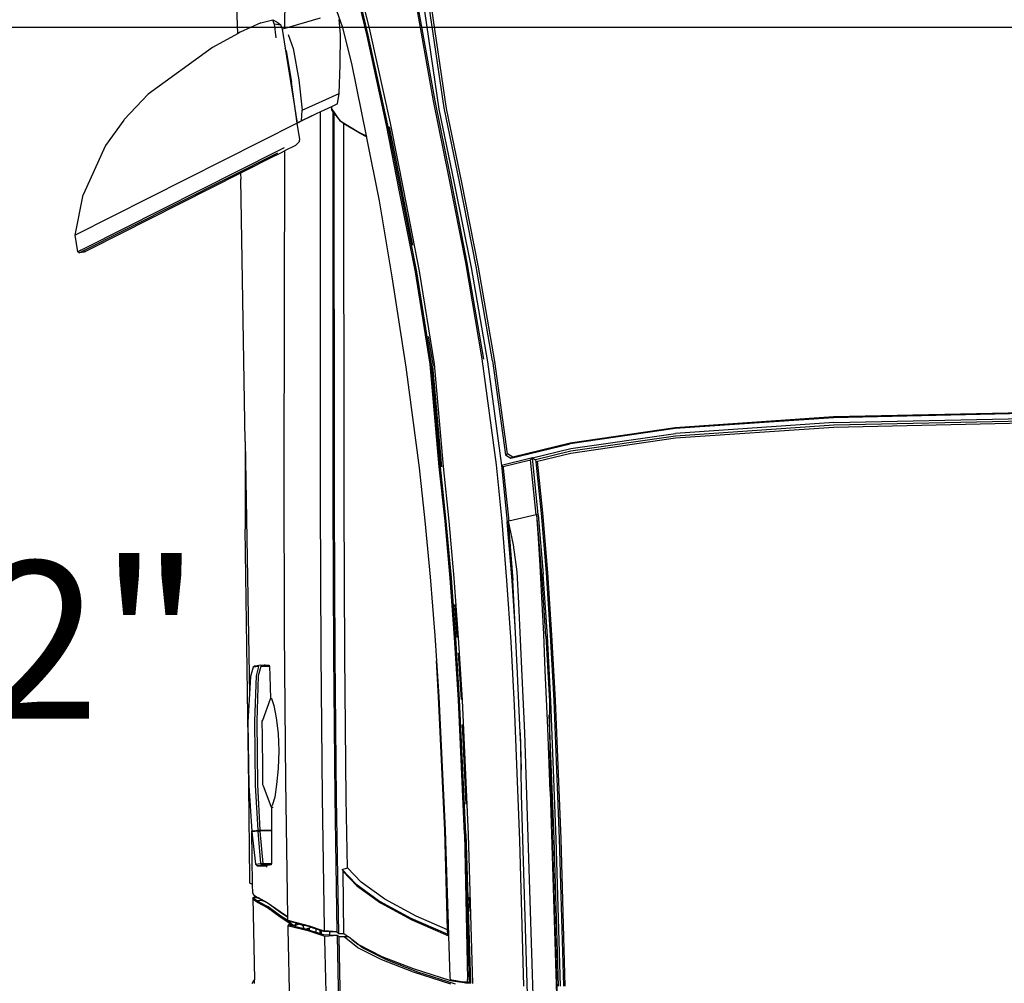
# Model space of a CAD drawing. Units: inches. Extents: x 1319 to 2030, y 219 to 1069.
# Tile 10 of 28: x 1417 to 1461, y 430 to 473. Entities that reach past the tile are written whole.
import ezdxf

# ---------------------------------------------------------------- set-up
doc = ezdxf.new("R2010")
doc.units = ezdxf.units.IN
doc.header["$MEASUREMENT"] = 0
doc.layers.get('0').update_dxf_attribs({"color": 12})
doc.layers.add('A-ANNO-DIMS', color=2, linetype='Continuous', lineweight=18)
doc.layers.add('C-PRKG-VEHC', color=8, linetype='Continuous', lineweight=13)
doc.layers.add('Edges', color=250, linetype='Continuous')
doc.styles.get("Standard").update_dxf_attribs({"font": 'arial.ttf'})
doc.dimstyles.get("Standard").update_dxf_attribs({"dimtxt": 7, "dimasz": 0.18, "dimexe": 0.18, "dimexo": 0.0625, "dimgap": 0.09, "dimtad": 0, "dimtih": 1, "dimtoh": 1, "dimzin": 0, "dimdsep": 46, "dimlunit": 3, "dimtxsty": 'Standard', "dimcen": 0.09, "dimadec": 0, "dimazin": 0, "dimtfac": 1, "dimtofl": 0, "dimtmove": 0, "dimatfit": 3, "dimfxl": 1, "dimtolj": 1, "dimtzin": 0, "dimarcsym": 0})

# ---------------------------------------------------------------- blocks, each defined once
blk = doc.blocks.new('Nissan Qashqai pl')
at = {"layer": 'Edges'}
for p, q in [((9.2195, 11.9221), (9.2241, 11.7066)), ((9.2203, 11.9221), (9.2249, 11.7065)), ((9.2305, 11.7067), (9.2259, 11.9221)), ((9.2289, 11.9221), (9.2335, 11.7067)), ((9.2355, 11.7068), (9.2308, 11.9221)), ((9.2241, 11.7066), (9.2362, 11.5274)), ((9.2249, 11.7065), (9.2371, 11.5273)), ((9.2305, 11.7067), (9.2426, 11.5277)), ((9.2335, 11.7067), (9.2457, 11.5277)), ((9.2476, 11.5278), (9.2355, 11.7068)), ((9.2362, 11.5274), (9.2535, 11.4087)), ((9.2371, 11.5273), (9.2543, 11.4085)), ((9.2598, 11.4093), (9.2426, 11.5277)), ((9.2457, 11.5277), (9.2629, 11.4092)), ((9.2649, 11.4094), (9.2476, 11.5278)), ((9.2535, 11.4087), (9.2694, 11.3436)), ((9.2707, 11.3414), (9.2543, 11.4085)), ((9.2704, 11.3659), (9.2598, 11.4093)), ((9.2629, 11.4092), (9.2726, 11.3695)), ((9.2741, 11.3716), (9.2649, 11.4094)), ((9.701, 11.3983), (9.5443, 11.3919)), ((9.5446, 11.39), (9.7011, 11.3963)), ((9.7014, 11.3929), (9.5454, 11.3866)), ((9.6472, 11.3861), (9.9278, 11.3949)), ((9.6714, 11.3874), (9.8565, 11.3931)), ((9.8673, 11.4031), (9.701, 11.3983)), ((9.7011, 11.3963), (9.8673, 11.4012)), ((9.8673, 11.3977), (9.7014, 11.3929)), ((9.8673, 11.3954), (9.7014, 11.3906)), ((9.8565, 11.3931), (9.9794, 11.3967)), ((9.4, 11.3832), (9.3326, 11.3776)), ((9.333, 11.3757), (9.4004, 11.3813)), ((9.4706, 11.388), (9.4, 11.3832)), ((9.4004, 11.3813), (9.4709, 11.3861)), ((9.472, 11.3812), (9.4017, 11.3765)), ((9.472, 11.3828), (9.4018, 11.378)), ((9.5443, 11.3919), (9.4706, 11.388)), ((9.4709, 11.3861), (9.5446, 11.39)), ((9.5454, 11.3866), (9.472, 11.3828)), ((9.472, 11.3812), (9.5454, 11.3851)), ((9.5755, 11.3834), (9.5105, 11.3805)), ((9.5454, 11.3851), (9.5695, 11.3853)), ((9.5454, 11.3848), (9.5454, 11.3851)), ((9.5695, 11.3853), (9.5609, 11.3849)), ((9.7014, 11.3906), (9.5695, 11.3853)), ((9.5695, 11.3853), (9.5786, 11.3853)), ((9.6472, 11.3861), (9.5755, 11.3834)), ((9.5786, 11.3853), (9.6206, 11.3861)), ((9.6206, 11.3861), (9.6714, 11.3874)), ((9.3346, 11.3724), (9.2704, 11.3659)), ((9.3346, 11.37), (9.2724, 11.3637)), ((9.3326, 11.3776), (9.2741, 11.3716)), ((9.2746, 11.3697), (9.333, 11.3757)), ((9.4017, 11.3765), (9.3344, 11.3708)), ((9.3611, 11.3727), (9.3344, 11.3708)), ((9.3344, 11.3708), (9.3346, 11.37)), ((9.3346, 11.3724), (9.4018, 11.378)), ((9.3346, 11.37), (9.3418, 11.3391)), ((9.3918, 11.3747), (9.3611, 11.3727)), ((9.4276, 11.3767), (9.3918, 11.3747)), ((9.4694, 11.3788), (9.4276, 11.3767)), ((9.5105, 11.3805), (9.4694, 11.3788)), ((9.2704, 11.3659), (9.2726, 11.3695)), ((9.2704, 11.3659), (9.2724, 11.3637)), ((9.2704, 11.3659), (9.2789, 11.331)), ((9.2799, 11.3328), (9.2724, 11.3637)), ((9.2726, 11.3695), (9.2746, 11.3697)), ((9.5812, 11.3568), (9.6514, 11.3592)), ((9.9583, 11.363), (9.651, 11.3536)), ((9.6514, 11.3592), (9.9312, 11.3681)), ((9.3687, 11.3441), (9.3992, 11.3482)), ((9.3992, 11.3482), (9.4347, 11.3502)), ((9.4347, 11.3502), (9.4761, 11.3522)), ((9.514, 11.3492), (9.4605, 11.3465)), ((9.4761, 11.3522), (9.5168, 11.3539)), ((9.5811, 11.3522), (9.514, 11.3492)), ((9.5168, 11.3539), (9.5812, 11.3568)), ((9.7029, 11.3516), (9.5503, 11.3455)), ((9.5811, 11.3522), (9.6231, 11.3531)), ((9.594, 11.3527), (9.5811, 11.3522)), ((9.6231, 11.3531), (9.594, 11.3527)), ((9.651, 11.3536), (9.6231, 11.3531)), ((9.8673, 11.3563), (9.7029, 11.3516)), ((9.2656, 11.3376), (9.1612, 11.3233)), ((9.2694, 11.3436), (9.2656, 11.3376)), ((9.2669, 11.3354), (9.2656, 11.3376)), ((9.2669, 11.3354), (9.2707, 11.3414)), ((9.2694, 11.3436), (9.2707, 11.3414)), ((9.2789, 11.331), (9.3427, 11.3375)), ((9.2819, 11.333), (9.3418, 11.3391)), ((9.3418, 11.3391), (9.342, 11.3383)), ((9.342, 11.3383), (9.3687, 11.3441)), ((9.342, 11.3383), (9.4087, 11.3438)), ((9.4088, 11.3371), (9.3422, 11.3316)), ((9.4093, 11.3431), (9.3427, 11.3375)), ((9.4605, 11.3465), (9.4087, 11.3438)), ((9.4782, 11.3418), (9.4088, 11.3371)), ((9.4605, 11.3465), (9.4093, 11.3431)), ((9.5503, 11.3455), (9.4782, 11.3418)), ((9.1605, 11.3208), (9.2669, 11.3354)), ((9.1617, 11.315), (9.2789, 11.331)), ((9.3422, 11.3316), (9.2783, 11.3251)), ((9.2789, 11.331), (9.2799, 11.3327)), ((9.2799, 11.3328), (9.2819, 11.333)), ((9.2799, 11.3327), (9.2799, 11.3328)), ((9.2799, 11.3327), (9.2811, 11.3325)), ((9.1605, 11.3208), (9.0538, 11.3023)), ((9.1612, 11.3233), (9.0546, 11.3048)), ((9.0552, 11.2965), (9.1617, 11.315)), ((9.2783, 11.3251), (9.1584, 11.3091)), ((9.0546, 11.3048), (8.9591, 11.2859)), ((9.1584, 11.3091), (9.0495, 11.2906)), ((9.0497, 11.2918), (9.1586, 11.3104)), ((9.0538, 11.3023), (8.9583, 11.2833)), ((8.9598, 11.2775), (9.0552, 11.2965)), ((9.5443, 11.2863), (9.696, 11.2932)), ((9.6953, 11.2892), (9.863, 11.2944)), ((9.6953, 11.2892), (9.8598, 11.2925)), ((9.6954, 11.2907), (9.8641, 11.2959)), ((9.696, 11.2932), (9.8644, 11.2982)), ((9.7669, 11.2945), (9.7832, 11.2951)), ((9.8629, 11.2925), (9.8598, 11.2925)), ((9.8627, 11.2909), (9.8629, 11.2925)), ((9.8629, 11.2925), (9.863, 11.2944)), ((9.8641, 11.2959), (9.863, 11.2944)), ((9.8637, 11.291), (9.8638, 11.2934)), ((9.8638, 11.2934), (9.8641, 11.2959)), ((8.9583, 11.2833), (8.8745, 11.266)), ((8.9591, 11.2859), (8.8754, 11.2687)), ((9.0495, 11.2906), (8.9521, 11.2715)), ((8.9522, 11.2728), (9.0497, 11.2918)), ((9.4064, 11.277), (9.4739, 11.282)), ((9.5437, 11.2822), (9.4735, 11.2779)), ((9.5438, 11.2836), (9.4736, 11.2793)), ((9.4739, 11.282), (9.5443, 11.2863)), ((9.491, 11.2819), (9.5434, 11.2852)), ((9.6953, 11.2892), (9.5437, 11.2822)), ((9.6954, 11.2907), (9.5438, 11.2836)), ((9.5717, 11.2865), (9.6618, 11.2907)), ((9.8605, 11.2746), (9.8626, 11.2878)), ((9.8615, 11.2754), (9.8635, 11.2886)), ((9.8626, 11.2878), (9.8627, 11.2909)), ((9.8627, 11.2909), (9.8637, 11.291)), ((9.8635, 11.2886), (9.8637, 11.291)), ((9.8637, 11.291), (9.8643, 11.291)), ((8.8666, 11.2554), (8.9522, 11.2728)), ((8.9521, 11.2715), (8.8666, 11.2541)), ((8.8761, 11.2602), (8.9598, 11.2775)), ((9.2801, 11.2648), (9.3418, 11.2713)), ((9.3418, 11.2713), (9.4064, 11.277)), ((9.4062, 11.2729), (9.3418, 11.2671)), ((9.4063, 11.2743), (9.3419, 11.2685)), ((9.4735, 11.2779), (9.4062, 11.2729)), ((9.4736, 11.2793), (9.4063, 11.2743)), ((9.4727, 11.2808), (9.4362, 11.278)), ((9.4727, 11.2808), (9.4732, 11.2808)), ((9.8039, 11.27), (9.6912, 11.2667)), ((9.6913, 11.2674), (9.8099, 11.2711)), ((9.8039, 11.27), (9.7884, 11.2343)), ((9.7905, 11.2283), (9.8087, 11.2702)), ((9.7925, 11.2294), (9.8107, 11.2711)), ((9.8087, 11.2702), (9.8039, 11.27)), ((9.8099, 11.2711), (9.8087, 11.2702)), ((9.8099, 11.2711), (9.8107, 11.2711)), ((9.8107, 11.2711), (9.8573, 11.2726)), ((9.8475, 11.2312), (9.8611, 11.2734)), ((9.8652, 11.2788), (9.8516, 11.2363)), ((9.8652, 11.2738), (9.8516, 11.2313)), ((9.8573, 11.2726), (9.8603, 11.2727)), ((9.8603, 11.2727), (9.8605, 11.2746)), ((9.8611, 11.2734), (9.8603, 11.2727)), ((9.8612, 11.2735), (9.8611, 11.2734)), ((9.8612, 11.2735), (9.8615, 11.2754)), ((8.8745, 11.266), (8.7481, 11.2473)), ((8.8754, 11.2687), (8.7491, 11.2501)), ((8.7496, 11.2416), (8.8761, 11.2602)), ((9.1639, 11.2546), (9.2801, 11.2648)), ((9.2803, 11.2606), (9.1644, 11.2503)), ((9.2804, 11.262), (9.1645, 11.2518)), ((9.2804, 11.2635), (9.1668, 11.2533)), ((9.3418, 11.2671), (9.2803, 11.2606)), ((9.3419, 11.2685), (9.2804, 11.262)), ((9.4997, 11.2573), (9.5403, 11.26)), ((9.5404, 11.2598), (9.4997, 11.2573)), ((9.5403, 11.26), (9.6913, 11.2674)), ((9.6912, 11.2667), (9.5404, 11.2598)), ((8.7287, 11.2307), (8.8666, 11.2554)), ((8.8666, 11.2541), (8.7292, 11.2295)), ((9.0591, 11.2377), (9.1639, 11.2546)), ((9.1644, 11.2503), (9.06, 11.2335)), ((9.1645, 11.2518), (9.0601, 11.235)), ((9.133, 11.2481), (9.1647, 11.2532)), ((9.1647, 11.2532), (9.1668, 11.2533)), ((9.3416, 11.2442), (9.4048, 11.2501)), ((9.4048, 11.2501), (9.471, 11.2554)), ((9.471, 11.2554), (9.4997, 11.2573)), ((8.9679, 11.2201), (9.0591, 11.2377)), ((9.1676, 11.2229), (9.2814, 11.2377)), ((9.2814, 11.2377), (9.3416, 11.2442)), ((9.0601, 11.235), (8.8941, 11.2023)), ((9.06, 11.2335), (8.9696, 11.2157)), ((8.9708, 11.2185), (9.03, 11.2304)), ((9.7884, 11.2343), (9.7692, 11.1989)), ((9.7713, 11.1929), (9.7905, 11.2283)), ((9.7733, 11.194), (9.7925, 11.2294)), ((9.8338, 11.1956), (9.8475, 11.2312)), ((9.8516, 11.2363), (9.8378, 11.2007)), ((9.8516, 11.2313), (9.8378, 11.1957)), ((8.8918, 11.205), (8.9679, 11.2201)), ((8.9696, 11.2157), (8.8942, 11.2009)), ((8.9318, 11.211), (8.9704, 11.2185)), ((8.9704, 11.2185), (8.9708, 11.2185)), ((9.0656, 11.207), (9.1676, 11.2229)), ((8.7881, 11.1821), (8.8918, 11.205)), ((8.8961, 11.204), (8.9318, 11.211)), ((8.9797, 11.1924), (9.0656, 11.207)), ((8.8941, 11.2023), (8.7925, 11.1802)), ((8.8942, 11.2009), (8.7931, 11.1789)), ((8.9087, 11.1783), (8.9797, 11.1924)), ((9.7692, 11.1989), (9.7499, 11.1721)), ((9.7519, 11.1661), (9.7713, 11.1929)), ((9.754, 11.1672), (9.7733, 11.194)), ((9.8201, 11.1685), (9.8338, 11.1956)), ((9.8378, 11.2007), (9.8241, 11.1736)), ((9.8378, 11.1957), (9.8241, 11.1686)), ((8.7575, 11.1744), (8.7881, 11.1821)), ((8.7931, 11.1789), (8.7574, 11.1704)), ((8.7925, 11.1802), (8.7591, 11.1723)), ((8.8245, 11.1613), (8.9063, 11.1779)), ((8.8893, 11.1486), (8.9021, 11.1697)), ((8.9041, 11.1717), (8.8927, 11.1528)), ((8.9021, 11.1697), (8.9063, 11.1779)), ((8.9075, 11.1781), (8.9041, 11.1717)), ((8.9063, 11.1779), (8.9075, 11.1781)), ((8.9075, 11.1781), (8.9087, 11.1783)), ((9.7499, 11.1721), (9.7337, 11.1566)), ((9.8241, 11.1736), (9.8147, 11.1616)), ((8.7828, 11.1508), (8.8245, 11.1613)), ((9.7357, 11.1507), (9.7519, 11.1661)), ((9.7378, 11.1517), (9.754, 11.1672)), ((9.8241, 11.1686), (9.8119, 11.1529)), ((9.8147, 11.1616), (9.8119, 11.1579)), ((9.8147, 11.1616), (9.8201, 11.1685)), ((9.8147, 11.1616), (9.8147, 11.1616)), ((8.7524, 11.1401), (8.7828, 11.1508)), ((8.7916, 11.1488), (8.7748, 11.1475)), ((8.8259, 11.1483), (8.7916, 11.1488)), ((8.8585, 11.1473), (8.8259, 11.1483)), ((8.87, 11.1455), (8.8585, 11.1473)), ((8.8771, 11.1054), (8.8585, 11.1473)), ((8.8893, 11.1486), (8.8751, 11.1387)), ((8.881, 11.1418), (8.8893, 11.1486)), ((8.8913, 11.1506), (8.8893, 11.1486)), ((8.8927, 11.1528), (8.8913, 11.1506)), ((9.3225, 11.1531), (8.8927, 11.1528)), ((9.4936, 11.1538), (9.3225, 11.1531)), ((9.6552, 11.1554), (9.4936, 11.1538)), ((9.7337, 11.1566), (9.6552, 11.1554)), ((9.7357, 11.1507), (9.7337, 11.1566)), ((9.7357, 11.1507), (9.7378, 11.1517)), ((9.8078, 11.1528), (9.7378, 11.1517)), ((9.8078, 11.1528), (9.8119, 11.1579)), ((9.8078, 11.1471), (9.8078, 11.1528)), ((9.8101, 11.1449), (9.9411, 11.1475)), ((9.8119, 11.1579), (9.8119, 11.1529)), ((9.8119, 11.1529), (9.8119, 11.1472)), ((9.9393, 11.1497), (9.8119, 11.1472)), ((8.87, 11.1455), (8.8734, 11.1385)), ((8.8734, 11.1385), (8.8793, 11.1261)), ((8.8734, 11.1385), (8.8768, 11.1385)), ((8.8751, 11.1387), (8.8768, 11.1385)), ((8.8768, 11.1385), (8.879, 11.1402)), ((8.879, 11.1402), (8.881, 11.1418)), ((8.879, 11.1402), (9.3198, 11.1403)), ((9.3225, 11.1421), (8.881, 11.1418)), ((9.3198, 11.1403), (9.4922, 11.1409)), ((9.4936, 11.1428), (9.3225, 11.1421)), ((9.4922, 11.1409), (9.654, 11.1423)), ((9.6552, 11.1445), (9.4936, 11.1428)), ((9.654, 11.1423), (9.8061, 11.1447)), ((9.8078, 11.1471), (9.6552, 11.1445)), ((9.8061, 11.1447), (9.8051, 11.1309)), ((9.8055, 11.1298), (9.8058, 11.1369)), ((9.8058, 11.1369), (9.8061, 11.1447)), ((9.8098, 11.1369), (9.8058, 11.1369)), ((9.8061, 11.1447), (9.8078, 11.1471)), ((9.8098, 11.1369), (9.8096, 11.13)), ((9.8101, 11.1449), (9.8098, 11.1369)), ((9.8119, 11.1472), (9.8101, 11.1449)), ((9.8101, 11.1449), (9.8112, 11.1311)), ((8.7733, 11.126), (8.7849, 11.0859)), ((9.3194, 11.1262), (8.8793, 11.1261)), ((8.8793, 11.1261), (8.8815, 11.1214)), ((9.4919, 11.1269), (9.3194, 11.1262)), ((9.6538, 11.1284), (9.4919, 11.1269)), ((9.802, 11.1309), (9.6538, 11.1284)), ((9.7992, 11.1133), (9.8044, 11.129)), ((9.8051, 11.1309), (9.802, 11.1309)), ((9.8026, 11.1212), (9.8041, 11.1256)), ((9.8041, 11.1256), (9.8045, 11.1268)), ((9.8041, 11.1256), (9.8081, 11.1256)), ((9.8044, 11.129), (9.8051, 11.1309)), ((9.8045, 11.1268), (9.8046, 11.1271)), ((9.8045, 11.1268), (9.8085, 11.1268)), ((9.8046, 11.1271), (9.8055, 11.1298)), ((9.8086, 11.1271), (9.8046, 11.1271)), ((9.8106, 11.1292), (9.8054, 11.1135)), ((9.8081, 11.1256), (9.8067, 11.1213)), ((9.8085, 11.1268), (9.8081, 11.1256)), ((9.8086, 11.1271), (9.8085, 11.1268)), ((9.8096, 11.13), (9.8086, 11.1271)), ((9.8112, 11.1311), (9.8106, 11.1292)), ((9.8143, 11.1312), (9.8112, 11.1311)), ((9.9414, 11.1341), (9.8143, 11.1312)), ((8.8815, 11.1214), (8.892, 11.0998)), ((8.8815, 11.1214), (8.8895, 11.1048)), ((9.7987, 11.108), (9.8002, 11.1141)), ((9.8002, 11.1141), (9.8008, 11.1157)), ((9.8008, 11.1157), (9.8014, 11.1176)), ((9.8014, 11.1139), (9.8008, 11.1157)), ((9.803, 11.1212), (9.8014, 11.1176)), ((9.8014, 11.1176), (9.8026, 11.1212)), ((9.8043, 11.1139), (9.8014, 11.1139)), ((9.8031, 11.1093), (9.8014, 11.1139)), ((9.803, 11.1212), (9.8026, 11.1212)), ((9.8067, 11.1213), (9.803, 11.1212)), ((9.8043, 11.1139), (9.8031, 11.1093)), ((9.8044, 11.1142), (9.8043, 11.1139)), ((9.8067, 11.1213), (9.8044, 11.1142)), ((8.8429, 11.1016), (8.8771, 11.1054)), ((8.8895, 11.1048), (8.8771, 11.1054)), ((8.8908, 11.1021), (8.8895, 11.1048)), ((8.8906, 11.1024), (8.8895, 11.1048)), ((8.9106, 11.1029), (8.892, 11.0998)), ((8.9131, 11.102), (8.9106, 11.1029)), ((9.7937, 11.0918), (9.7992, 11.1133)), ((9.7973, 11.1023), (9.7977, 11.1042)), ((9.7977, 11.1033), (9.7973, 11.1023)), ((9.7987, 11.1053), (9.7977, 11.1033)), ((9.7977, 11.1042), (9.7978, 11.1044)), ((9.7977, 11.1042), (9.7977, 11.1033)), ((9.7978, 11.1044), (9.7987, 11.108)), ((9.7987, 11.1053), (9.7978, 11.1044)), ((9.7992, 11.1065), (9.7987, 11.108)), ((9.7992, 11.1065), (9.7987, 11.1053)), ((9.8027, 11.1078), (9.7992, 11.1065)), ((9.8054, 11.1135), (9.7999, 11.0919)), ((9.8027, 11.1078), (9.8003, 11.0983)), ((9.8031, 11.1093), (9.8027, 11.1078)), ((8.7917, 11.0895), (8.8075, 11.0955)), ((8.807, 11.0862), (8.8918, 11.0997)), ((8.8075, 11.0955), (8.8429, 11.1016)), ((8.8102, 11.0874), (8.8455, 11.0936)), ((8.8918, 11.0997), (8.8455, 11.0936)), ((8.8906, 11.1024), (8.8911, 11.1013)), ((8.892, 11.0998), (8.8908, 11.1021)), ((8.8911, 11.1013), (8.8919, 11.0997)), ((8.8911, 11.1013), (8.8919, 11.0998)), ((8.8919, 11.0997), (8.8911, 11.1013)), ((8.8919, 11.0997), (8.8918, 11.0997)), ((8.8918, 11.0997), (9.0186, 10.8486)), ((8.892, 11.0998), (8.8919, 11.0998)), ((8.8919, 11.0998), (8.8919, 11.0997)), ((8.8919, 11.0997), (8.8919, 11.0997)), ((8.892, 11.0998), (8.892, 11.0998)), ((8.9171, 11.0978), (8.9131, 11.102)), ((8.9171, 11.0978), (8.917, 11.0974)), ((8.9171, 11.0978), (8.9233, 11.0855)), ((9.7965, 11.0915), (9.7894, 11.0806)), ((9.7934, 11.0906), (9.7937, 11.0918)), ((9.7964, 11.0988), (9.7943, 11.0907)), ((9.7955, 11.0925), (9.7943, 11.0907)), ((9.7963, 11.0918), (9.7955, 11.0925)), ((9.7992, 11.0966), (9.7963, 11.0918)), ((9.7963, 11.0918), (9.7963, 11.0918)), ((9.7964, 11.0917), (9.7963, 11.0918)), ((9.7964, 11.0988), (9.7973, 11.1023)), ((9.7964, 11.0988), (9.7992, 11.0966)), ((9.7964, 11.0917), (9.7996, 11.0966)), ((9.7964, 11.0917), (9.7964, 11.0917)), ((9.7967, 11.0915), (9.7964, 11.0917)), ((9.7965, 11.0915), (9.7967, 11.0915)), ((9.7983, 11.0901), (9.7965, 11.0915)), ((9.7967, 11.0915), (9.7986, 11.0916)), ((9.7977, 11.0907), (9.7967, 11.0915)), ((9.7973, 11.1023), (9.7977, 11.1011)), ((9.7977, 11.1011), (9.7977, 11.0998)), ((9.7977, 11.1011), (9.7985, 11.099)), ((9.7977, 11.0998), (9.7985, 11.099)), ((9.7986, 11.0916), (9.7982, 11.0902)), ((9.7985, 11.099), (9.7989, 11.098)), ((9.7988, 11.0925), (9.7986, 11.0916)), ((9.7998, 11.0964), (9.7988, 11.0925)), ((9.7989, 11.098), (9.7998, 11.0976)), ((9.7998, 11.0976), (9.7992, 11.0966)), ((9.7999, 11.0919), (9.7993, 11.0891)), ((9.8002, 11.098), (9.7996, 11.0966)), ((9.8001, 11.0974), (9.7996, 11.0966)), ((9.7996, 11.0966), (9.7998, 11.0964)), ((9.8003, 11.0983), (9.7998, 11.0976)), ((9.8001, 11.0974), (9.7998, 11.0964)), ((9.8002, 11.098), (9.8001, 11.0974)), ((9.8003, 11.0983), (9.8002, 11.098)), ((9.8024, 11.0892), (9.9426, 11.0923)), ((8.7849, 11.0859), (8.7205, 11.0863)), ((8.7779, 11.0773), (8.7807, 11.0812)), ((8.7798, 11.0739), (8.7807, 11.0812)), ((8.7849, 11.0827), (8.7807, 11.0812)), ((8.7849, 11.0859), (8.7856, 11.0834)), ((8.7849, 11.0827), (8.7858, 11.0828)), ((8.7858, 11.0828), (8.7856, 11.0834)), ((8.7858, 11.0828), (8.807, 11.0862)), ((8.8102, 11.0874), (8.807, 11.0862)), ((8.9232, 11.0779), (8.9194, 11.0854)), ((8.9233, 11.0855), (9.2886, 11.0848)), ((8.925, 11.0821), (8.9233, 11.0855)), ((8.928, 11.0762), (8.925, 11.0821)), ((9.2886, 11.0848), (9.4673, 11.0852)), ((9.4673, 11.0852), (9.6358, 11.0866)), ((9.6358, 11.0866), (9.7887, 11.0889)), ((9.7728, 11.066), (9.7832, 11.0805)), ((9.7738, 11.067), (9.7842, 11.0814)), ((9.7883, 11.0815), (9.7778, 11.0671)), ((9.7894, 11.0806), (9.7788, 11.0661)), ((9.7832, 11.0805), (9.7887, 11.0889)), ((9.7842, 11.0814), (9.7891, 11.0889)), ((9.7933, 11.0892), (9.7883, 11.0815)), ((9.7887, 11.0889), (9.7891, 11.0889)), ((9.7891, 11.0889), (9.79, 11.0889)), ((9.79, 11.0889), (9.7931, 11.089)), ((9.7931, 11.089), (9.7934, 11.0906)), ((9.7931, 11.089), (9.7933, 11.0892)), ((9.7933, 11.0892), (9.7941, 11.0901)), ((9.7934, 11.0906), (9.7938, 11.0904)), ((9.7941, 11.0901), (9.7943, 11.0907)), ((9.7982, 11.0902), (9.7977, 11.0907)), ((9.7983, 11.0901), (9.7982, 11.0902)), ((9.7986, 11.0898), (9.7983, 11.0901)), ((9.7986, 11.0898), (9.7993, 11.0891)), ((9.7993, 11.0891), (9.8024, 11.0892)), ((8.7751, 11.0723), (8.7779, 11.0773)), ((8.7798, 11.0739), (8.7751, 11.0723)), ((8.7785, 11.0587), (8.7751, 11.0723)), ((8.7798, 11.0739), (8.7954, 11.0758)), ((9.0333, 10.8597), (8.9232, 11.0779)), ((9.0386, 10.8534), (8.9254, 11.0778)), ((8.928, 11.0762), (8.9483, 11.0359)), ((9.5168, 11.0691), (9.5423, 11.0696)), ((9.5422, 11.0706), (9.5422, 11.0716)), ((9.5422, 11.0706), (9.5424, 11.0707)), ((9.5423, 11.0696), (9.5422, 11.0706)), ((9.5426, 11.0695), (9.5423, 11.0696)), ((9.5424, 11.0707), (9.5503, 11.0736)), ((9.5426, 11.0695), (9.5424, 11.0707)), ((9.5667, 11.0609), (9.5426, 11.0695)), ((9.5503, 11.0736), (9.5641, 11.076)), ((9.5641, 11.076), (9.5818, 11.0782)), ((9.5818, 11.0782), (9.6016, 11.0791)), ((9.6016, 11.0791), (9.6215, 11.0782)), ((9.6215, 11.0782), (9.6395, 11.0766)), ((9.6395, 11.0766), (9.654, 11.0744)), ((9.6645, 11.0705), (9.6413, 11.0616)), ((9.654, 11.0744), (9.6633, 11.0715)), ((9.6633, 11.0715), (9.6645, 11.0705)), ((9.6655, 11.0708), (9.6645, 11.0705)), ((9.6655, 11.0728), (9.6655, 11.0708)), ((9.6655, 11.0708), (9.6911, 11.0709)), ((9.6911, 11.0709), (9.692, 11.0709)), ((9.6911, 11.0645), (9.6911, 11.0709)), ((9.692, 11.0709), (9.692, 11.0645)), ((9.692, 11.0709), (9.7287, 11.0708)), ((9.7287, 11.0708), (9.7305, 11.0704)), ((9.7288, 11.0609), (9.7287, 11.0708)), ((9.7305, 11.0704), (9.7313, 11.0644)), ((9.7305, 11.0704), (9.7306, 11.0607)), ((8.7785, 11.0587), (8.7891, 11.0353)), ((9.5037, 11.0635), (9.5045, 11.0628)), ((9.5044, 11.0586), (9.5045, 11.0628)), ((9.5052, 11.0524), (9.5044, 11.0586)), ((9.5045, 11.0683), (9.5063, 11.0687)), ((9.5045, 11.0628), (9.5045, 11.0683)), ((9.5063, 11.0687), (9.5061, 11.0586)), ((9.5061, 11.0586), (9.5167, 11.0559)), ((9.5063, 11.0687), (9.5168, 11.0691)), ((9.5678, 11.0604), (9.5667, 11.0609)), ((9.5846, 11.0606), (9.5678, 11.0604)), ((9.6236, 11.0609), (9.5846, 11.0606)), ((9.64, 11.0611), (9.6236, 11.0609)), ((9.6413, 11.0616), (9.64, 11.0611)), ((9.6912, 11.0631), (9.6911, 11.0645)), ((9.692, 11.0631), (9.6912, 11.0631)), ((9.6912, 11.0577), (9.6912, 11.0631)), ((9.692, 11.0645), (9.692, 11.0631)), ((9.692, 11.0631), (9.6921, 11.0578)), ((9.6921, 11.0578), (9.7288, 11.0609)), ((9.7288, 11.0588), (9.6922, 11.0556)), ((9.7288, 11.0588), (9.7288, 11.0609)), ((9.7288, 11.0609), (9.7306, 11.0607)), ((9.7306, 11.0607), (9.7288, 11.0588)), ((9.7296, 11.0527), (9.7288, 11.0588)), ((9.7306, 11.0607), (9.7314, 11.0547)), ((9.733, 11.066), (9.7313, 11.0644)), ((9.7314, 11.0547), (9.7313, 11.0644)), ((9.7674, 11.0557), (9.7728, 11.066)), ((9.7684, 11.0567), (9.7717, 11.0631)), ((9.7717, 11.0631), (9.7707, 11.0593)), ((9.7707, 11.0593), (9.7709, 11.0549)), ((9.7717, 11.0631), (9.7738, 11.067)), ((9.7778, 11.0671), (9.7724, 11.0568)), ((9.7788, 11.0661), (9.7734, 11.0558)), ((9.5052, 11.0524), (9.5069, 11.0501)), ((9.5168, 11.0537), (9.5061, 11.0564)), ((9.5061, 11.0564), (9.5069, 11.0501)), ((9.5069, 11.0501), (9.5176, 11.0469)), ((9.5167, 11.0559), (9.5679, 11.0543)), ((9.5679, 11.0521), (9.5168, 11.0537)), ((9.5679, 11.0543), (9.64, 11.0549)), ((9.6401, 11.0528), (9.5679, 11.0521)), ((9.64, 11.0549), (9.6912, 11.0577)), ((9.6913, 11.0556), (9.6401, 11.0528)), ((9.641, 11.045), (9.6921, 11.0485)), ((9.6913, 11.0556), (9.6912, 11.0577)), ((9.692, 11.0499), (9.6913, 11.0556)), ((9.6922, 11.0499), (9.692, 11.0499)), ((9.6921, 11.0485), (9.692, 11.0499)), ((9.6922, 11.0556), (9.6921, 11.0578)), ((9.6922, 11.0499), (9.6921, 11.0485)), ((9.7526, 11.0495), (9.6921, 11.0485)), ((9.6922, 11.0556), (9.693, 11.0486)), ((9.6922, 11.0556), (9.6922, 11.0499)), ((9.693, 11.0486), (9.7296, 11.0527)), ((9.7296, 11.0527), (9.7314, 11.0547)), ((9.7526, 11.0495), (9.7511, 11.0463)), ((9.7623, 11.0497), (9.7526, 11.0495)), ((9.7623, 11.0497), (9.7643, 11.0504)), ((9.7643, 11.0504), (9.7652, 11.0514)), ((9.7643, 11.0504), (9.7648, 11.0513)), ((9.7648, 11.0513), (9.7664, 11.054)), ((9.7648, 11.0513), (9.7648, 11.0513)), ((9.7652, 11.0514), (9.7665, 11.0535)), ((9.7664, 11.054), (9.7674, 11.0557)), ((9.7665, 11.0537), (9.7664, 11.054)), ((9.7665, 11.0535), (9.7676, 11.0553)), ((9.7667, 11.0508), (9.7665, 11.0535)), ((9.7676, 11.0511), (9.7667, 11.0508)), ((9.7677, 11.0498), (9.7667, 11.0508)), ((9.7673, 11.0545), (9.7676, 11.0553)), ((9.7673, 11.0543), (9.7673, 11.0545)), ((9.7676, 11.0511), (9.7673, 11.0543)), ((9.7676, 11.0553), (9.7684, 11.0567)), ((9.7676, 11.0555), (9.7678, 11.056)), ((9.769, 11.0516), (9.7676, 11.0511)), ((9.7677, 11.0498), (9.8598, 11.0514)), ((9.77, 11.0506), (9.7677, 11.0498)), ((9.7677, 11.0498), (9.7677, 11.0498)), ((9.7712, 11.055), (9.769, 11.0516)), ((9.7734, 11.0558), (9.77, 11.0506)), ((9.7709, 11.0549), (9.7712, 11.055)), ((9.7724, 11.0568), (9.7712, 11.055)), ((9.8598, 11.0514), (9.8614, 11.0504)), ((9.8643, 11.0514), (9.8598, 11.0514)), ((9.8614, 11.0504), (9.8647, 11.0485)), ((8.9483, 11.0359), (8.9552, 11.0361)), ((8.9483, 11.0359), (9.0343, 10.8656)), ((9.2517, 11.0411), (8.9552, 11.0361)), ((9.2517, 11.0411), (9.5372, 11.0459)), ((9.2517, 11.0411), (9.351, 11.0411)), ((9.641, 11.045), (9.351, 11.0411)), ((9.5176, 11.0469), (9.5372, 11.0459)), ((9.5372, 11.0459), (9.5689, 11.0442)), ((9.5689, 11.0442), (9.641, 11.045)), ((9.7466, 11.0464), (9.641, 11.045)), ((9.7511, 11.0463), (9.7466, 11.0464)), ((8.7222, 11.0298), (8.7908, 11.0322)), ((8.7891, 11.0353), (8.7908, 11.0322)), ((8.7908, 11.0322), (8.8066, 11.0041)), ((8.8066, 11.0041), (8.8591, 10.9315)), ((8.8591, 10.9315), (8.8879, 10.9041)), ((8.8885, 10.9037), (8.8879, 10.9041)), ((8.8885, 10.9037), (8.9173, 10.8831)), ((8.9173, 10.8831), (8.9731, 10.8577)), ((9.0356, 10.8553), (9.0333, 10.8597)), ((9.0343, 10.8656), (9.0347, 10.8648)), ((9.0347, 10.8648), (9.0362, 10.8619)), ((9.0362, 10.8619), (9.037, 10.8603)), ((9.0371, 10.8601), (9.037, 10.8603)), ((9.0371, 10.8601), (9.0376, 10.8591)), ((9.0376, 10.8591), (9.0371, 10.8595)), ((9.0376, 10.8591), (9.0386, 10.8534)), ((9.0186, 10.8486), (8.9731, 10.8577)), ((9.0374, 10.8517), (9.0186, 10.8486)), ((9.0356, 10.8553), (9.0374, 10.8517)), ((9.0386, 10.8534), (9.0374, 10.8517))]:
    blk.add_line(p, q, dxfattribs=at)
blk = doc.blocks.new('car')
blk.add_blockref('Nissan Qashqai pl', (-9.7433, -11.9151))
blk = doc.blocks.new('carr')
blk.add_blockref('car', (0.5124, -0.007))
blk = doc.blocks.new('*D56')
at = {"layer": 'A-ANNO-DIMS', "color": 0, "lineweight": -2, "transparency": 16777216}
for p, q in [((1419.852, 531.201), (1393.865, 531.201)), ((1394.045, 531.021), (1394.045, 448.679)), ((1394.045, 358.918), (1394.045, 441.26)), ((1419.852, 358.738), (1393.865, 358.738))]:
    blk.add_line(p, q, dxfattribs=at)
at = {"layer": 'A-ANNO-DIMS', "color": 0, "transparency": 16777216}
for points in [[(1394.015, 531.021), (1394.075, 531.021), (1394.045, 531.201)], [(1394.015, 358.918), (1394.075, 358.918), (1394.045, 358.738)]]:
    blk.add_solid(points, dxfattribs=at)
at = {"layer": 'Defpoints', "color": 0, "transparency": 16777216}
for p in [(1419.914, 531.201), (1394.045, 358.738), (1419.914, 358.738)]:
    blk.add_point(p, dxfattribs=at)
at = {"layer": 'A-ANNO-DIMS', "color": 0, "transparency": 16777216, "insert": (1394.045, 444.969), "char_height": 7, "attachment_point": 5}
blk.add_mtext('\\A1;CAR 14\'-4 1/2"', dxfattribs=at)
blk = doc.blocks.new('*D65')
at = {"layer": 'A-ANNO-DIMS', "color": 0, "lineweight": -2, "transparency": 16777216}
for p, q in [((1648.280254, 472.227245), (1329.112754, 472.227245)), ((1329.292754, 472.047245), (1329.292754, 431.817245)), ((1329.292754, 384.407245), (1329.292754, 424.637245)), ((1648.280254, 384.227245), (1329.112754, 384.227245))]:
    blk.add_line(p, q, dxfattribs=at)
at = {"layer": 'A-ANNO-DIMS', "color": 0, "transparency": 16777216}
for points in [[(1329.262754, 472.047245), (1329.322754, 472.047245), (1329.292754, 472.227245)], [(1329.262754, 384.407245), (1329.322754, 384.407245), (1329.292754, 384.227245)]]:
    blk.add_solid(points, dxfattribs=at)
at = {"layer": 'Defpoints', "color": 0, "transparency": 16777216}
for p in [(1329.292754, 472.227245), (1648.342754, 472.227245), (1648.342754, 384.227245)]:
    blk.add_point(p, dxfattribs=at)
at = {"layer": 'A-ANNO-DIMS', "color": 0, "transparency": 16777216, "insert": (1329.292754, 428.227245), "char_height": 7, "attachment_point": 5}
blk.add_mtext('\\A1;7\'-4"', dxfattribs=at)

msp = doc.modelspace()

# ---------------------------------------------------------------- block references
at = {"layer": 'C-PRKG-VEHC', "xscale": 39.37007874015748, "yscale": 39.37007874015748, "zscale": 39.37007874015748, "rotation": 270}
msp.add_blockref('carr', (1462.179, 454.621), dxfattribs=at)

# ---------------------------------------------------------------- dimensions: what is measured, and where the dimension line sits
at = {"layer": 'A-ANNO-DIMS'}
dim = msp.add_linear_dim(base=(1394.045, 358.738), p1=(1419.914, 531.201), p2=(1419.914, 358.738), angle=270, text='CAR <>', dimstyle='Standard', override={"dimdec": 1, "dimlfac": 1, "dimrnd": 0, "dimzin": 1, "dimdsep": 46, "dimlunit": 4, "dimfrac": 2}, dxfattribs=at)
dim.commit()
dim.dimension.update_dxf_attribs({"geometry": '*D56', "text_midpoint": (1394.045, 444.969)})
dim = msp.add_linear_dim(base=(1329.293, 472.227), p1=(1648.343, 384.227), p2=(1648.343, 472.227), angle=90, dimstyle='Standard', override={"dimdec": 1, "dimlfac": 1, "dimrnd": 0, "dimzin": 1, "dimdsep": 46, "dimlunit": 4, "dimfrac": 2}, dxfattribs=at)
dim.commit()
dim.dimension.update_dxf_attribs({"geometry": '*D65', "text_midpoint": (1329.293, 428.227)})

doc.saveas('drawing.dxf')
